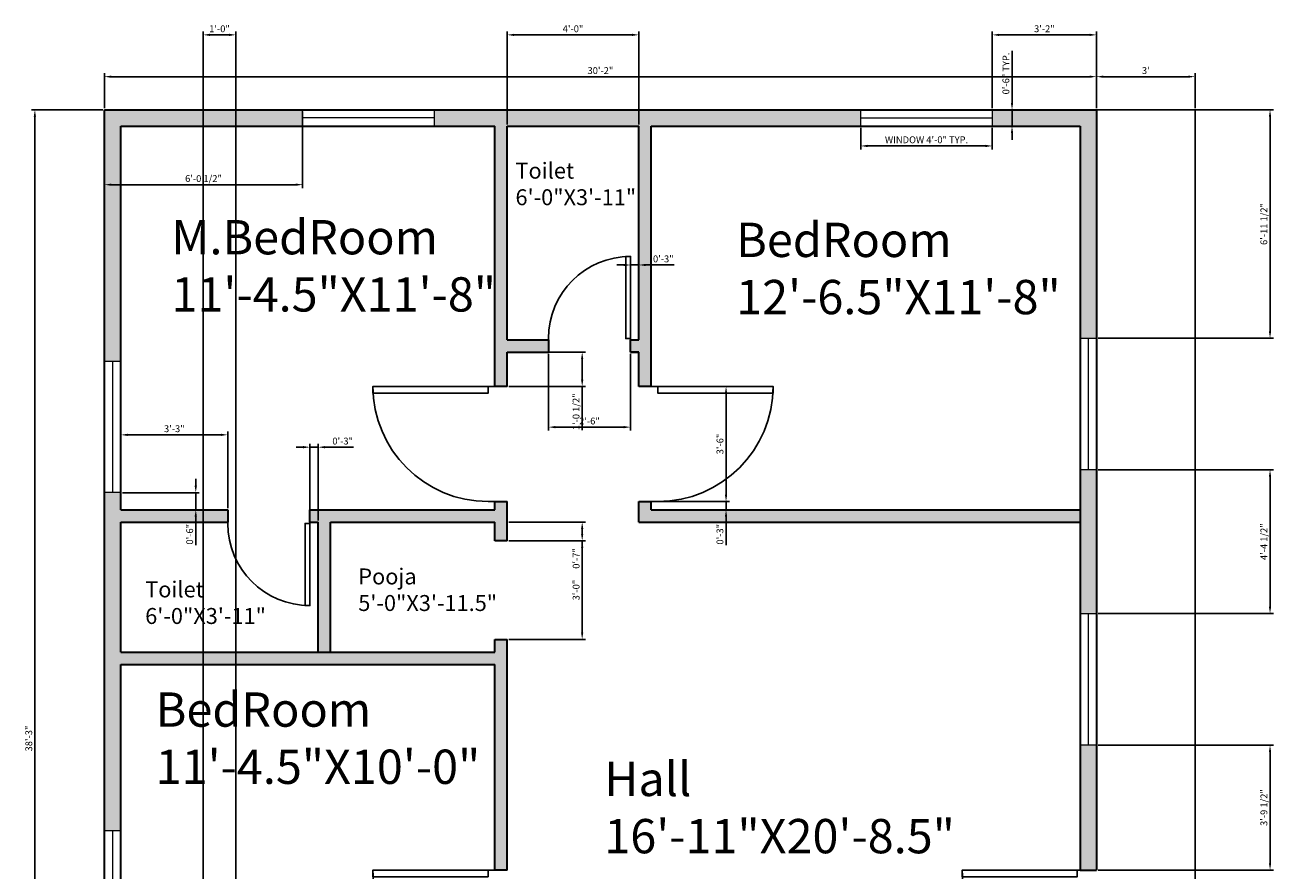
# Model space of a CAD drawing. Units: inches. Extents: x 1129603 to 1130059, y 1058961 to 1059552.
# Tile 2 of 2: x 1129603 to 1130059, y 1059243 to 1059552. Entities that reach past the tile are written whole.
import ezdxf

# ---------------------------------------------------------------- set-up
doc = ezdxf.new("R2010")
doc.units = ezdxf.units.IN
for name, color, linetype, lineweight in [('A-ANNO-DIMS', 2, 'Continuous', 18), ('A-AREA-IDEN', 7, 'Continuous', 25), ('A-DOOR', 3, 'Continuous', 25), ('A-GLAZ', 4, 'Continuous', 18), ('A-WALL-PATT', 9, 'Continuous', 13), ('C-PROP', 8, 'Continuous', 25), ('walls', 7, 'Continuous', 35)]:
    doc.layers.add(name, color=color, linetype=linetype, lineweight=lineweight)
doc.styles.get("Standard").update_dxf_attribs({"font": 'arial.ttf'})
doc.dimstyles.new('ISO-25', dxfattribs={"dimtxt": 2.5, "dimasz": 2.5, "dimexe": 1.25, "dimexo": 0.625, "dimtad": 1, "dimlunit": 4, "dimtxsty": 'Standard', "dimcen": 2.5, "dimadec": 0, "dimazin": 0, "dimtfac": 1, "dimtmove": 0, "dimatfit": 3, "dimfxl": 1, "dimarcsym": 0})

# ---------------------------------------------------------------- blocks, each defined once
blk = doc.blocks.new('*U2')
for p, q in [((0, 0), (0, -5)), ((30, 0), (30, -5))]:
    blk.add_line(p, q)
blk.add_lwpolyline([(0, 0), (0, 30), (1.75, 30), (1.75, 0)], close=True)
blk.add_arc((0, 0), 30, 0, 90)
blk = doc.blocks.new('*D3')
at = {"layer": 'A-ANNO-DIMS', "color": 0, "lineweight": -2, "transparency": 16777216}
for p, q in [((1129631.62, 1059521.5), (1129631.62, 1059534.21)), ((1129993.62, 1059521.5), (1129993.62, 1059534.21)), ((1129634.12, 1059532.96), (1129991.12, 1059532.96))]:
    blk.add_line(p, q, dxfattribs=at)
at = {"layer": 'A-ANNO-DIMS', "color": 0, "transparency": 16777216}
for points in [[(1129634.12, 1059533.37), (1129634.12, 1059532.54), (1129631.62, 1059532.96)], [(1129991.12, 1059533.37), (1129991.12, 1059532.54), (1129993.62, 1059532.96)]]:
    blk.add_solid(points, dxfattribs=at)
at = {"layer": 'Defpoints', "color": 0, "transparency": 16777216}
for p in [(1129993.62, 1059532.96), (1129631.62, 1059520.87), (1129993.62, 1059520.87)]:
    blk.add_point(p, dxfattribs=at)
at = {"layer": 'A-ANNO-DIMS', "color": 0, "transparency": 16777216, "insert": (1129812.62, 1059534.86), "char_height": 2.5, "attachment_point": 5}
blk.add_mtext('30\'-2"', dxfattribs=at)
blk = doc.blocks.new('*D4')
at = {"layer": 'A-ANNO-DIMS', "color": 0, "lineweight": -2, "transparency": 16777216}
for p, q in [((1129993.62, 1059521.5), (1129993.62, 1059534.21)), ((1130029.62, 1059521.5), (1130029.62, 1059534.21)), ((1129996.12, 1059532.96), (1130027.12, 1059532.96))]:
    blk.add_line(p, q, dxfattribs=at)
at = {"layer": 'A-ANNO-DIMS', "color": 0, "transparency": 16777216}
for points in [[(1129996.12, 1059533.37), (1129996.12, 1059532.54), (1129993.62, 1059532.96)], [(1130027.12, 1059533.37), (1130027.12, 1059532.54), (1130029.62, 1059532.96)]]:
    blk.add_solid(points, dxfattribs=at)
at = {"layer": 'Defpoints', "color": 0, "transparency": 16777216}
for p in [(1130029.62, 1059532.96), (1129993.62, 1059520.87), (1130029.62, 1059520.87)]:
    blk.add_point(p, dxfattribs=at)
at = {"layer": 'A-ANNO-DIMS', "color": 0, "transparency": 16777216, "insert": (1130011.62, 1059534.86), "char_height": 2.5, "attachment_point": 5}
blk.add_mtext("3'", dxfattribs=at)
blk = doc.blocks.new('*D5')
at = {"layer": 'A-ANNO-DIMS', "color": 0, "lineweight": -2, "transparency": 16777216}
for p, q in [((1129630.99, 1059520.87), (1129605, 1059520.87)), ((1129606.25, 1059518.37), (1129606.25, 1059064.37)), ((1129630.99, 1059061.87), (1129605, 1059061.87))]:
    blk.add_line(p, q, dxfattribs=at)
at = {"layer": 'A-ANNO-DIMS', "color": 0, "transparency": 16777216}
for points in [[(1129605.83, 1059518.37), (1129606.66, 1059518.37), (1129606.25, 1059520.87)], [(1129605.83, 1059064.37), (1129606.66, 1059064.37), (1129606.25, 1059061.87)]]:
    blk.add_solid(points, dxfattribs=at)
at = {"layer": 'Defpoints', "color": 0, "transparency": 16777216}
for p in [(1129631.62, 1059520.87), (1129606.25, 1059061.87), (1129631.62, 1059061.87)]:
    blk.add_point(p, dxfattribs=at)
at = {"layer": 'A-ANNO-DIMS', "color": 0, "transparency": 16777216, "insert": (1129604.34, 1059291.37), "char_height": 2.5, "attachment_point": 5, "rotation": 90}
blk.add_mtext('38\'-3"', dxfattribs=at)
blk = doc.blocks.new('WIN-48IN')
for p, q in [((0, 6), (48, 6)), ((0, 0), (0, 6)), ((48, 6), (48, 0)), ((0, 3), (48, 3)), ((48, 0), (0, 0))]:
    blk.add_line(p, q)
blk = doc.blocks.new('*D8')
at = {"layer": 'A-ANNO-DIMS', "color": 0, "lineweight": -2, "transparency": 16777216}
for p, q in [((1129907.61, 1059514.25), (1129907.61, 1059506.42)), ((1129955.61, 1059514.25), (1129955.61, 1059506.42)), ((1129910.11, 1059507.67), (1129953.11, 1059507.67))]:
    blk.add_line(p, q, dxfattribs=at)
at = {"layer": 'A-ANNO-DIMS', "color": 0, "transparency": 16777216}
for points in [[(1129910.11, 1059508.09), (1129910.11, 1059507.26), (1129907.61, 1059507.67)], [(1129953.11, 1059508.09), (1129953.11, 1059507.26), (1129955.61, 1059507.67)]]:
    blk.add_solid(points, dxfattribs=at)
at = {"layer": 'Defpoints', "color": 0, "transparency": 16777216}
for p in [(1129907.61, 1059514.87), (1129955.61, 1059514.87), (1129955.61, 1059507.67)]:
    blk.add_point(p, dxfattribs=at)
at = {"layer": 'A-ANNO-DIMS', "color": 0, "transparency": 16777216, "insert": (1129931.61, 1059509.59), "char_height": 2.5, "attachment_point": 5}
blk.add_mtext('WINDOW 4\'-0" TYP.', dxfattribs=at)
blk = doc.blocks.new('*D9')
at = {"layer": 'A-ANNO-DIMS', "color": 0, "lineweight": -2, "transparency": 16777216}
for p, q in [((1129962.81, 1059523.37), (1129962.81, 1059542.36)), ((1129956.23, 1059520.87), (1129964.06, 1059520.87)), ((1129962.81, 1059514.87), (1129962.81, 1059520.87)), ((1129956.23, 1059514.87), (1129964.06, 1059514.87)), ((1129962.81, 1059512.37), (1129962.81, 1059509.87))]:
    blk.add_line(p, q, dxfattribs=at)
at = {"layer": 'A-ANNO-DIMS', "color": 0, "transparency": 16777216}
for points in [[(1129962.39, 1059523.37), (1129963.23, 1059523.37), (1129962.81, 1059520.87)], [(1129962.39, 1059512.37), (1129963.23, 1059512.37), (1129962.81, 1059514.87)]]:
    blk.add_solid(points, dxfattribs=at)
at = {"layer": 'Defpoints', "color": 0, "transparency": 16777216}
for p in [(1129955.61, 1059520.87), (1129962.81, 1059520.87), (1129955.61, 1059514.87)]:
    blk.add_point(p, dxfattribs=at)
at = {"layer": 'A-ANNO-DIMS', "color": 0, "transparency": 16777216, "insert": (1129960.91, 1059534.12), "char_height": 2.5, "attachment_point": 5, "rotation": 90}
blk.add_mtext('0\'-6" TYP.', dxfattribs=at)
blk = doc.blocks.new('*D10')
at = {"layer": 'A-ANNO-DIMS', "color": 0, "lineweight": -2, "transparency": 16777216}
for p, q in [((1129631.62, 1059520.25), (1129631.62, 1059492.28)), ((1129703.95, 1059520.25), (1129703.95, 1059492.28)), ((1129701.45, 1059493.53), (1129634.12, 1059493.53))]:
    blk.add_line(p, q, dxfattribs=at)
at = {"layer": 'A-ANNO-DIMS', "color": 0, "transparency": 16777216}
for points in [[(1129634.12, 1059493.95), (1129634.12, 1059493.12), (1129631.62, 1059493.53)], [(1129701.45, 1059493.95), (1129701.45, 1059493.12), (1129703.95, 1059493.53)]]:
    blk.add_solid(points, dxfattribs=at)
at = {"layer": 'Defpoints', "color": 0, "transparency": 16777216}
for p in [(1129631.62, 1059520.87), (1129703.95, 1059520.87), (1129631.62, 1059493.53)]:
    blk.add_point(p, dxfattribs=at)
at = {"layer": 'A-ANNO-DIMS', "color": 0, "transparency": 16777216, "insert": (1129667.78, 1059495.45), "char_height": 2.5, "attachment_point": 5}
blk.add_mtext('6\'-0 1/2"', dxfattribs=at)
blk = doc.blocks.new('*D11')
at = {"layer": 'A-ANNO-DIMS', "color": 0, "lineweight": -2, "transparency": 16777216}
for p, q in [((1129955.61, 1059521.5), (1129955.61, 1059549.47)), ((1129958.11, 1059548.22), (1129991.12, 1059548.22)), ((1129993.62, 1059521.5), (1129993.62, 1059549.47))]:
    blk.add_line(p, q, dxfattribs=at)
at = {"layer": 'A-ANNO-DIMS', "color": 0, "transparency": 16777216}
for points in [[(1129958.11, 1059548.63), (1129958.11, 1059547.8), (1129955.61, 1059548.22)], [(1129991.12, 1059548.63), (1129991.12, 1059547.8), (1129993.62, 1059548.22)]]:
    blk.add_solid(points, dxfattribs=at)
at = {"layer": 'Defpoints', "color": 0, "transparency": 16777216}
for p in [(1129993.62, 1059548.22), (1129955.61, 1059520.87), (1129993.62, 1059520.87)]:
    blk.add_point(p, dxfattribs=at)
at = {"layer": 'A-ANNO-DIMS', "color": 0, "transparency": 16777216, "insert": (1129974.61, 1059550.12), "char_height": 2.5, "attachment_point": 5}
blk.add_mtext('3\'-2"', dxfattribs=at)
blk = doc.blocks.new('*D12')
at = {"layer": 'A-ANNO-DIMS', "color": 0, "lineweight": -2, "transparency": 16777216}
for p, q in [((1129664.96, 1059383.61), (1129664.96, 1059386.11)), ((1129638.24, 1059381.11), (1129666.21, 1059381.11)), ((1129664.96, 1059381.11), (1129664.96, 1059374.87)), ((1129638.24, 1059374.87), (1129666.21, 1059374.87)), ((1129664.96, 1059372.37), (1129664.96, 1059361.98))]:
    blk.add_line(p, q, dxfattribs=at)
at = {"layer": 'A-ANNO-DIMS', "color": 0, "transparency": 16777216}
for points in [[(1129664.54, 1059383.61), (1129665.37, 1059383.61), (1129664.96, 1059381.11)], [(1129664.54, 1059372.37), (1129665.37, 1059372.37), (1129664.96, 1059374.87)]]:
    blk.add_solid(points, dxfattribs=at)
at = {"layer": 'Defpoints', "color": 0, "transparency": 16777216}
for p in [(1129637.62, 1059381.11), (1129637.62, 1059374.87), (1129664.96, 1059374.87)]:
    blk.add_point(p, dxfattribs=at)
at = {"layer": 'A-ANNO-DIMS', "color": 0, "transparency": 16777216, "insert": (1129663.06, 1059365.93), "char_height": 2.5, "attachment_point": 5, "rotation": 90}
blk.add_mtext('0\'-6"', dxfattribs=at)
blk = doc.blocks.new('*D14')
at = {"layer": 'A-ANNO-DIMS', "color": 0, "lineweight": -2, "transparency": 16777216}
for p, q in [((1129994.24, 1059520.87), (1130058.21, 1059520.87)), ((1130056.96, 1059439.98), (1130056.96, 1059518.37)), ((1129994.24, 1059437.48), (1130058.21, 1059437.48))]:
    blk.add_line(p, q, dxfattribs=at)
at = {"layer": 'A-ANNO-DIMS', "color": 0, "transparency": 16777216}
for points in [[(1130056.54, 1059518.37), (1130057.37, 1059518.37), (1130056.96, 1059520.87)], [(1130056.54, 1059439.98), (1130057.37, 1059439.98), (1130056.96, 1059437.48)]]:
    blk.add_solid(points, dxfattribs=at)
at = {"layer": 'Defpoints', "color": 0, "transparency": 16777216}
for p in [(1129993.62, 1059520.87), (1130056.96, 1059520.87), (1129993.62, 1059437.48)]:
    blk.add_point(p, dxfattribs=at)
at = {"layer": 'A-ANNO-DIMS', "color": 0, "transparency": 16777216, "insert": (1130055.04, 1059479.18), "char_height": 2.5, "attachment_point": 5, "rotation": 90}
blk.add_mtext('6\'-11 1/2"', dxfattribs=at)
blk = doc.blocks.new('*D15')
at = {"layer": 'A-ANNO-DIMS', "color": 0, "lineweight": -2, "transparency": 16777216}
for p, q in [((1129994.24, 1059389.48), (1130058.21, 1059389.48)), ((1130056.96, 1059339.47), (1130056.96, 1059386.98)), ((1129994.24, 1059336.97), (1130058.21, 1059336.97))]:
    blk.add_line(p, q, dxfattribs=at)
at = {"layer": 'A-ANNO-DIMS', "color": 0, "transparency": 16777216}
for points in [[(1130056.54, 1059386.98), (1130057.37, 1059386.98), (1130056.96, 1059389.48)], [(1130056.54, 1059339.47), (1130057.37, 1059339.47), (1130056.96, 1059336.97)]]:
    blk.add_solid(points, dxfattribs=at)
at = {"layer": 'Defpoints', "color": 0, "transparency": 16777216}
for p in [(1129993.62, 1059389.48), (1130056.96, 1059389.48), (1129993.62, 1059336.97)]:
    blk.add_point(p, dxfattribs=at)
at = {"layer": 'A-ANNO-DIMS', "color": 0, "transparency": 16777216, "insert": (1130055.04, 1059363.22), "char_height": 2.5, "attachment_point": 5, "rotation": 90}
blk.add_mtext('4\'-4 1/2"', dxfattribs=at)
blk = doc.blocks.new('*D16')
at = {"layer": 'A-ANNO-DIMS', "color": 0, "lineweight": -2, "transparency": 16777216}
for p, q in [((1129994.24, 1059288.97), (1130058.21, 1059288.97)), ((1130056.96, 1059245.87), (1130056.96, 1059286.47)), ((1129994.24, 1059243.37), (1130058.21, 1059243.37))]:
    blk.add_line(p, q, dxfattribs=at)
at = {"layer": 'A-ANNO-DIMS', "color": 0, "transparency": 16777216}
for points in [[(1130056.54, 1059286.47), (1130057.37, 1059286.47), (1130056.96, 1059288.97)], [(1130056.54, 1059245.87), (1130057.37, 1059245.87), (1130056.96, 1059243.37)]]:
    blk.add_solid(points, dxfattribs=at)
at = {"layer": 'Defpoints', "color": 0, "transparency": 16777216}
for p in [(1129993.62, 1059288.97), (1130056.96, 1059288.97), (1129993.62, 1059243.37)]:
    blk.add_point(p, dxfattribs=at)
at = {"layer": 'A-ANNO-DIMS', "color": 0, "transparency": 16777216, "insert": (1130055.04, 1059266.17), "char_height": 2.5, "attachment_point": 5, "rotation": 90}
blk.add_mtext('3\'-9 1/2"', dxfattribs=at)
blk = doc.blocks.new('*D23')
at = {"layer": 'A-ANNO-DIMS', "color": 0, "lineweight": -2, "transparency": 16777216}
for p, q in [((1129667.62, 1058990.5), (1129667.62, 1059549.47)), ((1129670.12, 1059548.22), (1129677.12, 1059548.22)), ((1129679.62, 1058990.5), (1129679.62, 1059549.47))]:
    blk.add_line(p, q, dxfattribs=at)
at = {"layer": 'A-ANNO-DIMS', "color": 0, "transparency": 16777216}
for points in [[(1129670.12, 1059548.63), (1129670.12, 1059547.8), (1129667.62, 1059548.22)], [(1129677.12, 1059548.63), (1129677.12, 1059547.8), (1129679.62, 1059548.22)]]:
    blk.add_solid(points, dxfattribs=at)
at = {"layer": 'Defpoints', "color": 0, "transparency": 16777216}
for p in [(1129679.62, 1059548.22), (1129667.62, 1058989.87), (1129679.62, 1058989.87)]:
    blk.add_point(p, dxfattribs=at)
at = {"layer": 'A-ANNO-DIMS', "color": 0, "transparency": 16777216, "insert": (1129673.62, 1059550.12), "char_height": 2.5, "attachment_point": 5}
blk.add_mtext('1\'-0"', dxfattribs=at)
blk = doc.blocks.new('*D29')
at = {"layer": 'A-ANNO-DIMS', "color": 0, "lineweight": -2, "transparency": 16777216}
for p, q in [((1129831.74, 1059419.87), (1129859.71, 1059419.87)), ((1129858.46, 1059417.37), (1129858.46, 1059380.37)), ((1129831.74, 1059377.87), (1129859.71, 1059377.87))]:
    blk.add_line(p, q, dxfattribs=at)
at = {"layer": 'A-ANNO-DIMS', "color": 0, "transparency": 16777216}
for points in [[(1129858.04, 1059417.37), (1129858.87, 1059417.37), (1129858.46, 1059419.87)], [(1129858.04, 1059380.37), (1129858.87, 1059380.37), (1129858.46, 1059377.87)]]:
    blk.add_solid(points, dxfattribs=at)
at = {"layer": 'Defpoints', "color": 0, "transparency": 16777216}
for p in [(1129831.12, 1059419.87), (1129831.12, 1059377.87), (1129858.46, 1059377.87)]:
    blk.add_point(p, dxfattribs=at)
at = {"layer": 'A-ANNO-DIMS', "color": 0, "transparency": 16777216, "insert": (1129856.56, 1059398.87), "char_height": 2.5, "attachment_point": 5, "rotation": 90}
blk.add_mtext('3\'-6"', dxfattribs=at)
blk = doc.blocks.new('*D30')
at = {"layer": 'A-ANNO-DIMS', "color": 0, "lineweight": -2, "transparency": 16777216}
for p, q in [((1129793.62, 1059431.75), (1129793.62, 1059403.78)), ((1129823.62, 1059431.75), (1129823.62, 1059403.78)), ((1129821.12, 1059405.03), (1129796.12, 1059405.03))]:
    blk.add_line(p, q, dxfattribs=at)
at = {"layer": 'A-ANNO-DIMS', "color": 0, "transparency": 16777216}
for points in [[(1129796.12, 1059405.45), (1129796.12, 1059404.62), (1129793.62, 1059405.03)], [(1129821.12, 1059405.45), (1129821.12, 1059404.62), (1129823.62, 1059405.03)]]:
    blk.add_solid(points, dxfattribs=at)
at = {"layer": 'Defpoints', "color": 0, "transparency": 16777216}
for p in [(1129793.62, 1059432.37), (1129823.62, 1059432.37), (1129793.62, 1059405.03)]:
    blk.add_point(p, dxfattribs=at)
at = {"layer": 'A-ANNO-DIMS', "color": 0, "transparency": 16777216, "insert": (1129808.62, 1059406.93), "char_height": 2.5, "attachment_point": 5}
blk.add_mtext('2\'-6"', dxfattribs=at)
blk = doc.blocks.new('*D31')
at = {"layer": 'A-ANNO-DIMS', "color": 0, "lineweight": -2, "transparency": 16777216}
for p, q in [((1129779.24, 1059363.55), (1129807.21, 1059363.55)), ((1129805.96, 1059361.05), (1129805.96, 1059330.05)), ((1129779.24, 1059327.55), (1129807.21, 1059327.55))]:
    blk.add_line(p, q, dxfattribs=at)
at = {"layer": 'A-ANNO-DIMS', "color": 0, "transparency": 16777216}
for points in [[(1129805.54, 1059361.05), (1129806.37, 1059361.05), (1129805.96, 1059363.55)], [(1129805.54, 1059330.05), (1129806.37, 1059330.05), (1129805.96, 1059327.55)]]:
    blk.add_solid(points, dxfattribs=at)
at = {"layer": 'Defpoints', "color": 0, "transparency": 16777216}
for p in [(1129778.62, 1059363.55), (1129778.62, 1059327.55), (1129805.96, 1059327.55)]:
    blk.add_point(p, dxfattribs=at)
at = {"layer": 'A-ANNO-DIMS', "color": 0, "transparency": 16777216, "insert": (1129804.06, 1059345.55), "char_height": 2.5, "attachment_point": 5, "rotation": 90}
blk.add_mtext('3\'-0"', dxfattribs=at)
blk = doc.blocks.new('*D32')
at = {"layer": 'A-ANNO-DIMS', "color": 0, "lineweight": -2, "transparency": 16777216}
for p, q in [((1129858.46, 1059380.37), (1129858.46, 1059382.87)), ((1129831.74, 1059377.87), (1129859.71, 1059377.87)), ((1129831.74, 1059374.87), (1129859.71, 1059374.87)), ((1129858.46, 1059377.87), (1129858.46, 1059374.87)), ((1129858.46, 1059372.37), (1129858.46, 1059361.98))]:
    blk.add_line(p, q, dxfattribs=at)
at = {"layer": 'A-ANNO-DIMS', "color": 0, "transparency": 16777216}
for points in [[(1129858.04, 1059380.37), (1129858.87, 1059380.37), (1129858.46, 1059377.87)], [(1129858.04, 1059372.37), (1129858.87, 1059372.37), (1129858.46, 1059374.87)]]:
    blk.add_solid(points, dxfattribs=at)
at = {"layer": 'Defpoints', "color": 0, "transparency": 16777216}
for p in [(1129831.12, 1059377.87), (1129831.12, 1059374.87), (1129858.46, 1059374.87)]:
    blk.add_point(p, dxfattribs=at)
at = {"layer": 'A-ANNO-DIMS', "color": 0, "transparency": 16777216, "insert": (1129856.56, 1059365.93), "char_height": 2.5, "attachment_point": 5, "rotation": 90}
blk.add_mtext('0\'-3"', dxfattribs=at)
blk = doc.blocks.new('*D33')
at = {"layer": 'A-ANNO-DIMS', "color": 0, "lineweight": -2, "transparency": 16777216}
for p, q in [((1129823.62, 1059437.5), (1129823.62, 1059465.47)), ((1129826.62, 1059437.5), (1129826.62, 1059465.47)), ((1129821.12, 1059464.22), (1129818.62, 1059464.22)), ((1129823.62, 1059464.22), (1129826.62, 1059464.22)), ((1129829.12, 1059464.22), (1129839.51, 1059464.22))]:
    blk.add_line(p, q, dxfattribs=at)
at = {"layer": 'A-ANNO-DIMS', "color": 0, "transparency": 16777216}
for points in [[(1129821.12, 1059464.63), (1129821.12, 1059463.8), (1129823.62, 1059464.22)], [(1129829.12, 1059464.63), (1129829.12, 1059463.8), (1129826.62, 1059464.22)]]:
    blk.add_solid(points, dxfattribs=at)
at = {"layer": 'Defpoints', "color": 0, "transparency": 16777216}
for p in [(1129826.62, 1059464.22), (1129823.62, 1059436.87), (1129826.62, 1059436.87)]:
    blk.add_point(p, dxfattribs=at)
at = {"layer": 'A-ANNO-DIMS', "color": 0, "transparency": 16777216, "insert": (1129835.56, 1059466.12), "char_height": 2.5, "attachment_point": 5}
blk.add_mtext('0\'-3"', dxfattribs=at)
blk = doc.blocks.new('*D34')
at = {"layer": 'A-ANNO-DIMS', "color": 0, "lineweight": -2, "transparency": 16777216}
for p, q in [((1129637.62, 1059375.5), (1129637.62, 1059403.47)), ((1129640.12, 1059402.22), (1129674.12, 1059402.22)), ((1129676.62, 1059375.5), (1129676.62, 1059403.47))]:
    blk.add_line(p, q, dxfattribs=at)
at = {"layer": 'A-ANNO-DIMS', "color": 0, "transparency": 16777216}
for points in [[(1129640.12, 1059402.63), (1129640.12, 1059401.8), (1129637.62, 1059402.22)], [(1129674.12, 1059402.63), (1129674.12, 1059401.8), (1129676.62, 1059402.22)]]:
    blk.add_solid(points, dxfattribs=at)
at = {"layer": 'Defpoints', "color": 0, "transparency": 16777216}
for p in [(1129676.62, 1059402.22), (1129637.62, 1059374.87), (1129676.62, 1059374.87)]:
    blk.add_point(p, dxfattribs=at)
at = {"layer": 'A-ANNO-DIMS', "color": 0, "transparency": 16777216, "insert": (1129657.12, 1059404.12), "char_height": 2.5, "attachment_point": 5}
blk.add_mtext('3\'-3"', dxfattribs=at)
blk = doc.blocks.new('*D35')
at = {"layer": 'A-ANNO-DIMS', "color": 0, "lineweight": -2, "transparency": 16777216}
for p, q in [((1129779.24, 1059370.37), (1129807.21, 1059370.37)), ((1129805.96, 1059367.87), (1129805.96, 1059366.05)), ((1129779.24, 1059363.55), (1129807.21, 1059363.55)), ((1129805.96, 1059363.55), (1129805.96, 1059353.16))]:
    blk.add_line(p, q, dxfattribs=at)
at = {"layer": 'A-ANNO-DIMS', "color": 0, "transparency": 16777216}
for points in [[(1129805.54, 1059367.87), (1129806.37, 1059367.87), (1129805.96, 1059370.37)], [(1129805.54, 1059366.05), (1129806.37, 1059366.05), (1129805.96, 1059363.55)]]:
    blk.add_solid(points, dxfattribs=at)
at = {"layer": 'Defpoints', "color": 0, "transparency": 16777216}
for p in [(1129778.62, 1059370.37), (1129778.62, 1059363.55), (1129805.96, 1059363.55)]:
    blk.add_point(p, dxfattribs=at)
at = {"layer": 'A-ANNO-DIMS', "color": 0, "transparency": 16777216, "insert": (1129804.06, 1059357.11), "char_height": 2.5, "attachment_point": 5, "rotation": 90}
blk.add_mtext('0\'-7"', dxfattribs=at)
blk = doc.blocks.new('*D39')
at = {"layer": 'A-ANNO-DIMS', "color": 0, "lineweight": -2, "transparency": 16777216}
for p, q in [((1129779.24, 1059432.37), (1129807.21, 1059432.37)), ((1129805.96, 1059429.87), (1129805.96, 1059422.37)), ((1129779.24, 1059419.87), (1129807.21, 1059419.87)), ((1129805.96, 1059419.87), (1129805.96, 1059403.89))]:
    blk.add_line(p, q, dxfattribs=at)
at = {"layer": 'A-ANNO-DIMS', "color": 0, "transparency": 16777216}
for points in [[(1129805.54, 1059429.87), (1129806.37, 1059429.87), (1129805.96, 1059432.37)], [(1129805.54, 1059422.37), (1129806.37, 1059422.37), (1129805.96, 1059419.87)]]:
    blk.add_solid(points, dxfattribs=at)
at = {"layer": 'Defpoints', "color": 0, "transparency": 16777216}
for p in [(1129778.62, 1059432.37), (1129778.62, 1059419.87), (1129805.96, 1059419.87)]:
    blk.add_point(p, dxfattribs=at)
at = {"layer": 'A-ANNO-DIMS', "color": 0, "transparency": 16777216, "insert": (1129804.04, 1059410.63), "char_height": 2.5, "attachment_point": 5, "rotation": 90}
blk.add_mtext('1\'-0 1/2"', dxfattribs=at)
blk = doc.blocks.new('*D43')
at = {"layer": 'A-ANNO-DIMS', "color": 0, "lineweight": -2, "transparency": 16777216}
for p, q in [((1129778.62, 1059515.5), (1129778.62, 1059549.47)), ((1129781.12, 1059548.22), (1129824.12, 1059548.22)), ((1129826.62, 1059515.5), (1129826.62, 1059549.47))]:
    blk.add_line(p, q, dxfattribs=at)
at = {"layer": 'A-ANNO-DIMS', "color": 0, "transparency": 16777216}
for points in [[(1129781.12, 1059548.63), (1129781.12, 1059547.8), (1129778.62, 1059548.22)], [(1129824.12, 1059548.63), (1129824.12, 1059547.8), (1129826.62, 1059548.22)]]:
    blk.add_solid(points, dxfattribs=at)
at = {"layer": 'Defpoints', "color": 0, "transparency": 16777216}
for p in [(1129826.62, 1059548.22), (1129778.62, 1059514.87), (1129826.62, 1059514.87)]:
    blk.add_point(p, dxfattribs=at)
at = {"layer": 'A-ANNO-DIMS', "color": 0, "transparency": 16777216, "insert": (1129802.62, 1059550.12), "char_height": 2.5, "attachment_point": 5}
blk.add_mtext('4\'-0"', dxfattribs=at)
blk = doc.blocks.new('*D45')
at = {"layer": 'A-ANNO-DIMS', "color": 0, "lineweight": -2, "transparency": 16777216}
for p, q in [((1129704.12, 1059397.72), (1129701.62, 1059397.72)), ((1129706.62, 1059371), (1129706.62, 1059398.97)), ((1129706.62, 1059397.72), (1129709.62, 1059397.72)), ((1129709.62, 1059371), (1129709.62, 1059398.97)), ((1129712.12, 1059397.72), (1129722.51, 1059397.72))]:
    blk.add_line(p, q, dxfattribs=at)
at = {"layer": 'A-ANNO-DIMS', "color": 0, "transparency": 16777216}
for points in [[(1129704.12, 1059398.13), (1129704.12, 1059397.3), (1129706.62, 1059397.72)], [(1129712.12, 1059398.13), (1129712.12, 1059397.3), (1129709.62, 1059397.72)]]:
    blk.add_solid(points, dxfattribs=at)
at = {"layer": 'Defpoints', "color": 0, "transparency": 16777216}
for p in [(1129709.62, 1059397.72), (1129706.62, 1059370.37), (1129709.62, 1059370.37)]:
    blk.add_point(p, dxfattribs=at)
at = {"layer": 'A-ANNO-DIMS', "color": 0, "transparency": 16777216, "insert": (1129718.56, 1059399.62), "char_height": 2.5, "attachment_point": 5}
blk.add_mtext('0\'-3"', dxfattribs=at)

msp = doc.modelspace()

# ---------------------------------------------------------------- hatches: boundary and pattern name
at = {"layer": 'A-WALL-PATT'}
h = msp.add_hatch(color=256, dxfattribs=at)
h.dxf.hatch_style = 1
h.paths.add_polyline_path([(1129703.948, 1059520.874), (1129631.616, 1059520.874), (1129631.616, 1059429.113), (1129637.616, 1059429.113), (1129637.616, 1059514.874), (1129703.948, 1059514.874)])
h = msp.add_hatch(color=256, dxfattribs=at)
h.dxf.hatch_style = 1
h.paths.add_polyline_path([(1129907.61, 1059520.874), (1129751.948, 1059520.874), (1129751.948, 1059514.874), (1129774.116, 1059514.874), (1129774.116, 1059419.874), (1129778.616, 1059419.874), (1129778.616, 1059432.374), (1129793.616, 1059432.374), (1129793.616, 1059436.874), (1129778.616, 1059436.874), (1129778.616, 1059514.874), (1129826.616, 1059514.874), (1129826.616, 1059436.874), (1129823.616, 1059436.874), (1129823.616, 1059432.374), (1129826.616, 1059432.374), (1129826.616, 1059419.874), (1129831.116, 1059419.874), (1129831.116, 1059514.874), (1129907.61, 1059514.874)])
h = msp.add_hatch(color=256, dxfattribs=at)
h.dxf.hatch_style = 1
h.paths.add_polyline_path([(1129993.616, 1059520.874), (1129955.61, 1059520.874), (1129955.61, 1059514.874), (1129987.616, 1059514.874), (1129987.616, 1059437.482), (1129993.616, 1059437.482)])
h = msp.add_hatch(color=256, dxfattribs=at)
h.dxf.hatch_style = 1
h.paths.add_polyline_path([(1129993.616, 1059389.482), (1129987.616, 1059389.482), (1129987.616, 1059336.967), (1129993.616, 1059336.967)])
h = msp.add_hatch(color=256, dxfattribs=at)
h.dxf.hatch_style = 1
h.paths.add_polyline_path([(1129778.616, 1059327.554), (1129774.116, 1059327.554), (1129774.116, 1059322.874), (1129637.616, 1059322.874), (1129637.616, 1059370.374), (1129676.616, 1059370.374), (1129676.616, 1059374.874), (1129637.616, 1059374.874), (1129637.616, 1059381.113), (1129631.616, 1059381.113), (1129631.616, 1059257.837), (1129637.616, 1059257.837), (1129637.616, 1059318.374), (1129774.116, 1059318.374), (1129774.116, 1059243.374), (1129778.616, 1059243.374)])
h = msp.add_hatch(color=256, dxfattribs=at)
h.dxf.hatch_style = 1
h.paths.add_polyline_path([(1129778.616, 1059377.874), (1129774.116, 1059377.874), (1129774.116, 1059374.874), (1129706.616, 1059374.874), (1129706.616, 1059370.374), (1129709.616, 1059370.374), (1129709.616, 1059322.874), (1129714.116, 1059322.874), (1129714.116, 1059370.374), (1129774.116, 1059370.374), (1129774.116, 1059363.554), (1129778.616, 1059363.554), (1129778.616, 1059370.374)], flags=17)
h = msp.add_hatch(color=256, dxfattribs=at)
h.dxf.hatch_style = 1
h.paths.add_polyline_path([(1129987.616, 1059374.874), (1129831.116, 1059374.874), (1129831.116, 1059377.874), (1129826.616, 1059377.874), (1129826.616, 1059374.874), (1129826.616, 1059370.374), (1129987.616, 1059370.374)])
h = msp.add_hatch(color=256, dxfattribs=at)
h.dxf.hatch_style = 1
h.paths.add_polyline_path([(1129993.616, 1059288.967), (1129987.616, 1059288.967), (1129987.616, 1059243.374), (1129993.616, 1059243.374)])

# ---------------------------------------------------------------- linework, layer by layer
at = {"layer": 'C-PROP'}
for p, q in [((1129993.616, 1059520.874), (1130029.616, 1059520.874)), ((1130029.616, 1059520.874), (1130029.616, 1059061.874))]:
    msp.add_line(p, q, dxfattribs=at)
at = {"layer": 'walls'}
for p, q in [((1129631.616, 1059520.874), (1129993.616, 1059520.874)), ((1129631.616, 1059061.874), (1129631.616, 1059520.874)), ((1129993.616, 1059520.874), (1129993.616, 1059243.374)), ((1129637.616, 1059514.874), (1129774.116, 1059514.874)), ((1129637.616, 1059374.874), (1129637.616, 1059514.874)), ((1129774.116, 1059419.874), (1129774.116, 1059514.874)), ((1129778.616, 1059514.874), (1129826.616, 1059514.874)), ((1129778.616, 1059436.874), (1129778.616, 1059514.874)), ((1129826.616, 1059436.874), (1129826.616, 1059514.874)), ((1129831.116, 1059514.874), (1129987.616, 1059514.874)), ((1129831.116, 1059419.874), (1129831.116, 1059514.874)), ((1129987.616, 1059514.874), (1129987.616, 1059243.374)), ((1129778.616, 1059436.874), (1129793.616, 1059436.874)), ((1129793.616, 1059436.874), (1129793.616, 1059432.374)), ((1129823.616, 1059432.374), (1129823.616, 1059436.874)), ((1129823.616, 1059436.874), (1129826.616, 1059436.874)), ((1129778.616, 1059432.374), (1129793.616, 1059432.374)), ((1129778.616, 1059419.874), (1129778.616, 1059432.374)), ((1129826.616, 1059432.374), (1129823.616, 1059432.374)), ((1129823.616, 1059432.374), (1129826.616, 1059432.374)), ((1129826.616, 1059419.874), (1129826.616, 1059432.374)), ((1129778.616, 1059419.874), (1129774.116, 1059419.874)), ((1129831.116, 1059419.874), (1129826.616, 1059419.874)), ((1129637.616, 1059374.874), (1129676.616, 1059374.874)), ((1129676.616, 1059374.874), (1129676.616, 1059370.374)), ((1129706.616, 1059370.374), (1129706.616, 1059374.874)), ((1129706.616, 1059374.874), (1129774.116, 1059374.874)), ((1129774.116, 1059374.874), (1129774.116, 1059377.874)), ((1129774.116, 1059377.874), (1129778.616, 1059377.874)), ((1129778.616, 1059370.374), (1129778.616, 1059377.874)), ((1129826.616, 1059370.374), (1129826.616, 1059377.874)), ((1129826.616, 1059374.874), (1129826.616, 1059377.874)), ((1129826.616, 1059377.874), (1129831.116, 1059377.874)), ((1129831.116, 1059374.874), (1129831.116, 1059377.874)), ((1129831.116, 1059374.874), (1129987.616, 1059374.874)), ((1129637.616, 1059370.374), (1129676.616, 1059370.374)), ((1129637.616, 1059322.874), (1129637.616, 1059370.374)), ((1129706.616, 1059370.374), (1129709.616, 1059370.374)), ((1129709.616, 1059322.874), (1129709.616, 1059370.374)), ((1129714.116, 1059322.874), (1129714.116, 1059370.374)), ((1129714.116, 1059370.374), (1129774.116, 1059370.374)), ((1129774.116, 1059363.554), (1129774.116, 1059370.374)), ((1129778.616, 1059363.554), (1129778.616, 1059370.374)), ((1129826.616, 1059370.374), (1129987.616, 1059370.374)), ((1129778.616, 1059363.554), (1129774.116, 1059363.554)), ((1129774.116, 1059322.874), (1129774.116, 1059327.554)), ((1129774.116, 1059327.554), (1129778.616, 1059327.554)), ((1129778.616, 1059243.374), (1129778.616, 1059327.554)), ((1129637.616, 1059322.874), (1129774.116, 1059322.874)), ((1129637.616, 1059198.374), (1129637.616, 1059318.374)), ((1129637.616, 1059318.374), (1129774.116, 1059318.374)), ((1129774.116, 1059243.374), (1129774.116, 1059318.374)), ((1129778.616, 1059243.374), (1129774.116, 1059243.374)), ((1129987.616, 1059243.374), (1129993.616, 1059243.374))]:
    msp.add_line(p, q, dxfattribs=at)

# ---------------------------------------------------------------- block references
at = {"layer": 'A-DOOR', "xscale": -1}
msp.add_blockref('*U2', (1129823.616, 1059437.374), dxfattribs=at)
at = {"layer": 'A-DOOR', "yscale": 1.399999999999999, "zscale": 1.399999999999999}
for p, xscale, rotation in [((1129771.616, 1059419.874), -1.399999999999999, 90), ((1129833.616, 1059419.874), 1.399999999999999, 270), ((1129771.616, 1059243.374), -1.399999999999999, 90), ((1129986.616, 1059243.374), -1.399999999999999, 90)]:
    msp.add_blockref('*U2', p, dxfattribs=dict(at, xscale=xscale, rotation=rotation))
at = {"layer": 'A-DOOR', "rotation": 180}
msp.add_blockref('*U2', (1129706.616, 1059369.874), dxfattribs=at)
at = {"layer": 'A-GLAZ'}
for p, rotation in [((1129751.948, 1059520.874), 180), ((1129987.616, 1059437.482), 270.0000000001367), ((1129631.616, 1059429.113), 269.9999999996579), ((1129987.616, 1059336.967), 270.0000000001367), ((1129631.616, 1059257.837), 269.9999999996579)]:
    msp.add_blockref('WIN-48IN', p, dxfattribs=dict(at, rotation=rotation))
msp.add_blockref('WIN-48IN', (1129907.61, 1059514.874), dxfattribs=at)

# ---------------------------------------------------------------- texts
at = {"layer": 'A-AREA-IDEN', "attachment_point": 1}
for s, width, gutter_width, insert, char_height in [('Toilet\\P6\'-0"X3\'-11"', 9.32652, 29.105, (1129781.615, 1059501.559), 5.82097), ('M.BedRoom\\P11\'-4.5"X11\'-8"', 31.97186, 62.607, (1129656.069, 1059480.615), 12.52132), ('BedRoom\\P12\'-6.5"X11\'-8"', 31.97186, 62.607, (1129862.133, 1059479.644), 12.52132), ('Pooja\\P5\'-0"X3\'-11.5"', 9.32652, 29.105, (1129724.253, 1059353.441), 5.82097), ('Toilet\\P6\'-0"X3\'-11"', 9.32652, 29.105, (1129646.506, 1059348.713), 5.82097), ('BedRoom\\P11\'-4.5"X10\'-0"', 31.97186, 62.607, (1129650.321, 1059308.196), 12.52132), ('Hall\\P16\'-11"X20\'-8.5"', 31.97186, 62.607, (1129814.028, 1059282.872), 12.52132)]:
    msp.add_mtext_dynamic_manual_height_columns(s, width=width, gutter_width=gutter_width, heights=[0], dxfattribs=dict(at, insert=insert, char_height=char_height))

# ---------------------------------------------------------------- dimensions: what is measured, and where the dimension line sits
at = {"layer": 'A-ANNO-DIMS'}
for base, p1, p2, override, picture, middle in [((1129679.616, 1059548.217), (1129667.616, 1058989.874), (1129679.616, 1058989.874), {"dimdec": 1, "dimlfac": 1, "dimrnd": 0, "dimzin": 1, "dimdsep": 46, "dimlunit": 4, "dimfrac": 2}, '*D23', (1129673.616, 1059550.118)), ((1129826.616, 1059548.217), (1129778.616, 1059514.874), (1129826.616, 1059514.874), {"dimdec": 1, "dimlfac": 1, "dimrnd": 0, "dimzin": 1, "dimdsep": 46, "dimlunit": 4, "dimfrac": 2}, '*D43', (1129802.616, 1059550.118)), ((1129993.616, 1059548.217), (1129955.61, 1059520.874), (1129993.616, 1059520.874), {"dimdec": 1, "dimlfac": 1, "dimrnd": 0, "dimzin": 1, "dimdsep": 46, "dimlunit": 4, "dimfrac": 2}, '*D11', (1129974.613, 1059550.119)), ((1129993.616, 1059532.957), (1129631.616, 1059520.874), (1129993.616, 1059520.874), {"dimclrd": 0, "dimclre": 0, "dimclrt": 0}, '*D3', (1129812.616, 1059534.86)), ((1130029.616, 1059532.957), (1129993.616, 1059520.874), (1130029.616, 1059520.874), {"dimclrd": 0, "dimclre": 0, "dimclrt": 0}, '*D4', (1130011.616, 1059534.86)), ((1129826.616, 1059464.217), (1129823.616, 1059436.874), (1129826.616, 1059436.874), {"dimdec": 1, "dimlfac": 1, "dimrnd": 0, "dimzin": 1, "dimdsep": 46, "dimlunit": 4, "dimfrac": 2}, '*D33', (1129835.564, 1059466.119)), ((1129676.616, 1059402.217), (1129637.616, 1059374.874), (1129676.616, 1059374.874), {"dimdec": 1, "dimlfac": 1, "dimrnd": 0, "dimzin": 1, "dimdsep": 46, "dimlunit": 4, "dimfrac": 2}, '*D34', (1129657.116, 1059404.119)), ((1129709.616, 1059397.717), (1129706.616, 1059370.374), (1129709.616, 1059370.374), {"dimdec": 1, "dimlfac": 1, "dimrnd": 0, "dimzin": 1, "dimdsep": 46, "dimlunit": 4, "dimfrac": 2}, '*D45', (1129718.564, 1059399.619))]:
    dim = msp.add_linear_dim(base=base, p1=p1, p2=p2, dimstyle='ISO-25', override=override, dxfattribs=at)
    dim.commit()
    dim.dimension.update_dxf_attribs({"geometry": picture, "text_midpoint": middle})
dim = msp.add_linear_dim(base=(1129962.81, 1059520.874), p1=(1129955.61, 1059514.874), p2=(1129955.61, 1059520.874), angle=90, text='<> TYP.', dimstyle='ISO-25', override={"dimdec": 1, "dimlfac": 1, "dimrnd": 0, "dimzin": 1, "dimdsep": 46, "dimlunit": 4, "dimfrac": 2}, dxfattribs=at)
dim.commit()
dim.dimension.update_dxf_attribs({"geometry": '*D9', "text_midpoint": (1129960.908, 1059534.119)})
for base, p1, p2, angle, override, picture, middle in [((1129606.247, 1059061.874), (1129631.616, 1059520.874), (1129631.616, 1059061.874), 90, {"dimclrd": 0, "dimclre": 0, "dimclrt": 0}, '*D5', (1129604.345, 1059291.374)), ((1129631.616, 1059493.532), (1129703.948, 1059520.874), (1129631.616, 1059520.874), 180, {"dimdec": 1, "dimlfac": 1, "dimrnd": 0, "dimzin": 1, "dimdsep": 46, "dimlunit": 4, "dimfrac": 2}, '*D10', (1129667.782, 1059495.449)), ((1130056.958, 1059520.874), (1129993.616, 1059437.482), (1129993.616, 1059520.874), 90, {"dimdec": 1, "dimlfac": 1, "dimrnd": 0, "dimzin": 1, "dimdsep": 46, "dimlunit": 4, "dimfrac": 2}, '*D14', (1130055.041, 1059479.178)), ((1129805.958, 1059419.874), (1129778.616, 1059432.374), (1129778.616, 1059419.874), 270, {"dimdec": 1, "dimlfac": 1, "dimrnd": 0, "dimzin": 1, "dimdsep": 46, "dimlunit": 4, "dimfrac": 2}, '*D39', (1129804.041, 1059410.631)), ((1129793.616, 1059405.032), (1129823.616, 1059432.374), (1129793.616, 1059432.374), 180, {"dimdec": 1, "dimlfac": 1, "dimrnd": 0, "dimzin": 1, "dimdsep": 46, "dimlunit": 4, "dimfrac": 2}, '*D30', (1129808.616, 1059406.933)), ((1129858.458, 1059377.874), (1129831.116, 1059419.874), (1129831.116, 1059377.874), 270, {"dimdec": 1, "dimlfac": 1, "dimrnd": 0, "dimzin": 1, "dimdsep": 46, "dimlunit": 4, "dimfrac": 2}, '*D29', (1129856.556, 1059398.874)), ((1130056.958, 1059389.482), (1129993.616, 1059336.967), (1129993.616, 1059389.482), 90, {"dimdec": 1, "dimlfac": 1, "dimrnd": 0, "dimzin": 1, "dimdsep": 46, "dimlunit": 4, "dimfrac": 2}, '*D15', (1130055.041, 1059363.224)), ((1129664.958, 1059374.874), (1129637.616, 1059381.113), (1129637.616, 1059374.874), 270, {"dimdec": 1, "dimlfac": 1, "dimrnd": 0, "dimzin": 1, "dimdsep": 46, "dimlunit": 4, "dimfrac": 2}, '*D12', (1129663.057, 1059365.926)), ((1129858.458, 1059374.874), (1129831.116, 1059377.874), (1129831.116, 1059374.874), 270, {"dimdec": 1, "dimlfac": 1, "dimrnd": 0, "dimzin": 1, "dimdsep": 46, "dimlunit": 4, "dimfrac": 2}, '*D32', (1129856.556, 1059365.926)), ((1129805.958, 1059363.554), (1129778.616, 1059370.374), (1129778.616, 1059363.554), 270, {"dimdec": 1, "dimlfac": 1, "dimrnd": 0, "dimzin": 1, "dimdsep": 46, "dimlunit": 4, "dimfrac": 2}, '*D35', (1129804.057, 1059357.106)), ((1129805.958, 1059327.554), (1129778.616, 1059363.554), (1129778.616, 1059327.554), 270, {"dimdec": 1, "dimlfac": 1, "dimrnd": 0, "dimzin": 1, "dimdsep": 46, "dimlunit": 4, "dimfrac": 2}, '*D31', (1129804.056, 1059345.554)), ((1130056.958, 1059288.967), (1129993.616, 1059243.374), (1129993.616, 1059288.967), 90, {"dimdec": 1, "dimlfac": 1, "dimrnd": 0, "dimzin": 1, "dimdsep": 46, "dimlunit": 4, "dimfrac": 2}, '*D16', (1130055.04, 1059266.171))]:
    dim = msp.add_linear_dim(base=base, p1=p1, p2=p2, angle=angle, dimstyle='ISO-25', override=override, dxfattribs=at)
    dim.commit()
    dim.dimension.update_dxf_attribs({"geometry": picture, "text_midpoint": middle})
dim = msp.add_linear_dim(base=(1129955.61, 1059507.674), p1=(1129907.61, 1059514.874), p2=(1129955.61, 1059514.874), text='WINDOW <> TYP.', dimstyle='ISO-25', override={"dimdec": 1, "dimlfac": 1, "dimrnd": 0, "dimzin": 1, "dimdsep": 46, "dimlunit": 4, "dimfrac": 2}, dxfattribs=at)
dim.commit()
dim.dimension.update_dxf_attribs({"geometry": '*D8', "text_midpoint": (1129931.61, 1059509.593)})

doc.saveas('drawing.dxf')
